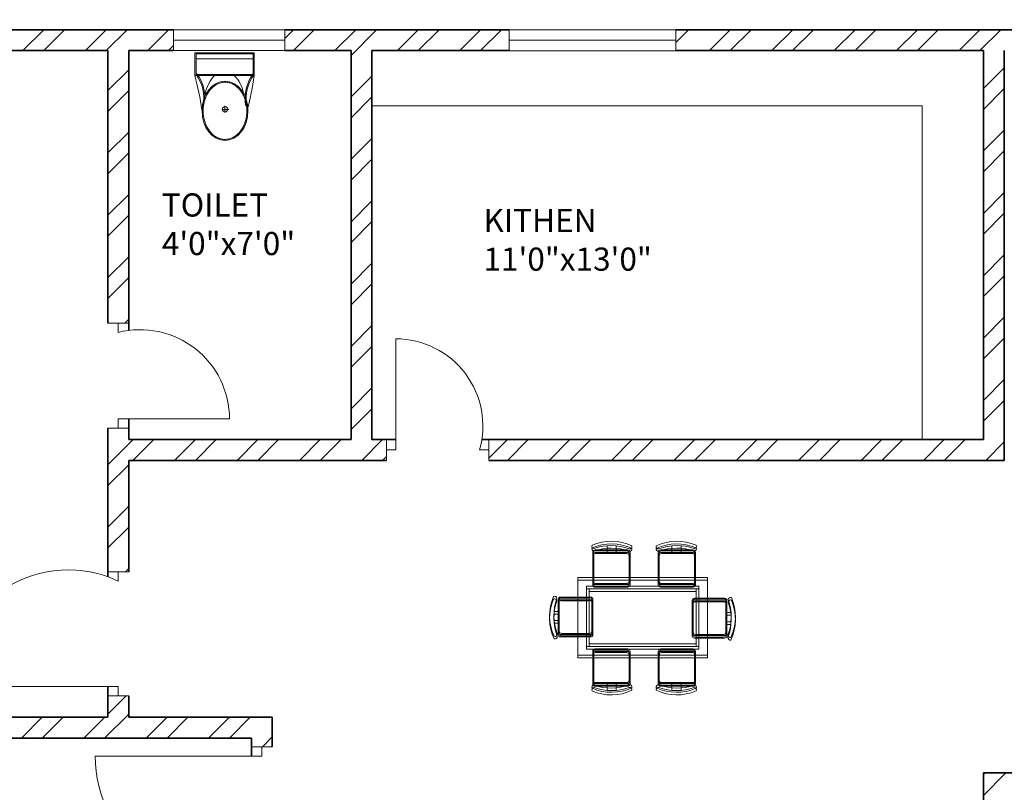
# Model space of a CAD drawing. Units: inches. Extents: x 1885 to 2748, y 783 to 2421.
# Tile 49 of 117: x 2098 to 2311, y 1683 to 1850. Entities that reach past the tile are written whole.
import ezdxf

# ---------------------------------------------------------------- set-up
doc = ezdxf.new("R2010")
doc.units = ezdxf.units.IN
for name, color, linetype, lineweight in [('A-AREA-IDEN', 7, 'Continuous', 18), ('A-DOOR', 31, 'Continuous', 18), ('A-FLOR-CASE', 9, 'Continuous', 18), ('A-FLOR-FIXT', 8, 'Continuous', 18), ('A-FURN', 8, 'Continuous', 13), ('A-GLAZ', 181, 'Continuous', 18), ('A-WALL', 7, 'Continuous', 35)]:
    doc.layers.add(name, color=color, linetype=linetype, lineweight=lineweight)
doc.layers.add('A-WALL-PATT', color=85, linetype='Continuous', lineweight=13, true_color=0x58ba48)
doc.styles.get("Standard").update_dxf_attribs({"font": 'arial.ttf'})

# ---------------------------------------------------------------- blocks, each defined once
blk = doc.blocks.new('A$C31115884')
for p, q in [((257.5, 466.4), (257.5, 523.2)), ((283.1, 497.7), (223.4, 497.7)), ((0, 200), (0, 0)), ((520, 200), (0, 200)), ((10, 190), (10, 10)), ((510, 190), (10, 190)), ((510, 10), (510, 190)), ((520, 0), (520, 200)), ((510, 54.5), (0, 54.5)), ((10, 10), (510, 10)), ((0, 0), (520, 0))]:
    blk.add_line(p, q)
blk.add_circle((255.6, 496.4), 23.6)
for centre, radius, start, end in [((2777.7, -204.6), 2807, 165.4549, 171.71327), ((-294.5, 403.3), 364.7, 324.20913, 9.34987), ((-294.5, 403.3), 374.7, 324.20913, 9.34987), ((805.8, 403.3), 364.7, 170.65013, 215.79087), ((3237, 905), 2807, 188.28673, 194.5451), ((383.6, 406.2), 293.5, 190.27735, 224.15636), ((139.5, 406.2), 293.5, 315.84364, 2.65635), ((805.8, 403.3), 374.7, 179.20365, 215.79087)]:
    blk.add_arc(centre, radius, start, end)
blk.add_ellipse((256.2, 509.9), major_axis=(0, -260.7), ratio=0.772727)
blk.add_open_spline([(256.2, 259.2), (263.1, 259.2), (270, 259.7), (287.8, 262.3), (298.7, 265.1), (319.9, 273.1), (330.2, 278.4), (350.1, 291.1), (359.7, 298.7), (377.7, 315.9), (386.2, 325.5), (401.7, 346.6), (408.8, 358.1), (421.3, 382.5), (426.8, 395.5), (435.9, 422.4), (439.5, 436.4), (444.8, 465.1), (446.5, 479.7), (447.9, 509.2), (447.6, 524), (445, 553.3), (442.7, 567.8), (436.3, 596), (432.1, 609.7), (421.9, 636), (416, 648.6), (402.5, 672.1), (395, 683), (378.6, 703), (369.8, 712.1), (351.1, 728), (341.3, 734.8), (320.9, 746.2), (310.4, 750.7), (288.9, 757.3), (278, 759.4), (256, 761), (245, 760.6), (223.1, 757.2), (212.3, 754.3), (191.1, 746.1), (180.8, 740.7), (160.9, 727.8), (151.4, 720.1), (133.5, 702.7), (125.1, 693), (109.6, 671.7), (102.6, 660.2), (90.2, 635.7), (84.9, 622.7), (76, 595.6), (72.4, 581.6), (67.2, 552.9), (65.6, 538.2), (64.4, 508.8), (64.8, 494), (67.5, 464.7), (69.9, 450.2), (76.6, 422), (80.8, 408.3), (91.1, 382.2), (97.2, 369.7), (110.8, 346.3), (118.4, 335.4), (134.8, 315.6), (143.7, 306.7), (162.4, 290.9), (172.3, 284.2), (192.8, 273), (203.3, 268.6), (224.8, 262.2), (235.8, 260.2), (249.9, 259.3), (253, 259.2), (256.2, 259.2)], degree=3, knots=[0, 0, 0, 0, 0.110105, 0.110105, 0.285049, 0.285049, 0.459994, 0.459994, 0.634938, 0.634938, 0.809882, 0.809882, 0.984827, 0.984827, 1.159771, 1.159771, 1.334715, 1.334715, 1.50966, 1.50966, 1.684604, 1.684604, 1.859549, 1.859549, 2.034493, 2.034493, 2.209437, 2.209437, 2.384382, 2.384382, 2.559326, 2.559326, 2.73427, 2.73427, 2.909215, 2.909215, 3.084159, 3.084159, 3.259103, 3.259103, 3.434048, 3.434048, 3.608992, 3.608992, 3.783936, 3.783936, 3.958881, 3.958881, 4.133825, 4.133825, 4.30877, 4.30877, 4.483714, 4.483714, 4.658658, 4.658658, 4.833603, 4.833603, 5.008547, 5.008547, 5.183491, 5.183491, 5.358436, 5.358436, 5.53338, 5.53338, 5.708324, 5.708324, 5.883269, 5.883269, 6.058213, 6.058213, 6.233158, 6.233158, 6.283185, 6.283185, 6.283185, 6.283185])
blk = doc.blocks.new('WIN-24')
for p, q in [((0, 4.5), (0, 0)), ((0, 4.5), (24, 4.5)), ((24, 2.25), (24, 4.5)), ((24, 4.5), (24, 0)), ((0, 0), (0, 2.25)), ((0, 2.25), (24, 2.25)), ((24, 0), (0, 0))]:
    blk.add_line(p, q)
blk = doc.blocks.new('WIN-36-ALT')
for p, q in [((0, 36), (4.5, 36)), ((0, 36), (0, 0)), ((4.5, 36), (2.25, 36)), ((2.25, 36), (2.25, 0)), ((4.5, 0), (4.5, 36)), ((4.5, 0), (0, 0)), ((2.25, 0), (4.5, 0))]:
    blk.add_line(p, q)

msp = doc.modelspace()

# ---------------------------------------------------------------- hatches: boundary and pattern name
at = {"layer": 'A-WALL-PATT'}
h = msp.add_hatch(dxfattribs=at)
h.set_pattern_fill('ANSI32', color=256)
h.paths.add_polyline_path([(2007.77, 2318.01), (1980.77, 2318.01), (1980.77, 2281.22), (1985.27, 2281.22), (1985.27, 2313.51), (2007.77, 2313.51), (2007.77, 2315.76)])
h.paths.add_polyline_path([(2094.32, 2318.01), (2067.77, 2318.01), (2067.77, 2313.51), (2094.32, 2313.51), (2094.32, 2315.76)])
h.paths.add_polyline_path([(2131.37, 2315.76), (2131.37, 2318.01), (2131.19, 2318.01), (2112.61, 2318.01), (2112.61, 2313.51), (2117.27, 2313.51), (2117.27, 2255.2), (2121.77, 2255.2), (2121.77, 2313.51), (2131.37, 2313.51)])
h.paths.add_polyline_path([(2190.51, 2318.01), (2155.37, 2318.01), (2155.37, 2313.51), (2169.77, 2313.51), (2169.77, 2229.51), (2121.77, 2229.51), (2121.77, 2233.45), (2119.52, 2233.45), (2117.27, 2233.45), (2117.27, 2201.1), (2121.77, 2201.1), (2121.77, 2225.01), (2169.77, 2225.01), (2169.77, 2165.01), (2306.27, 2165.01), (2306.27, 2066.01), (2310.77, 2066.01), (2344.27, 2066.01), (2486.27, 2066.01), (2486.27, 1886.01), (2483.02, 1886.01), (2483.02, 1881.51), (2486.27, 1881.51), (2486.27, 1880.68), (2490.77, 1880.68), (2490.77, 2070.51), (2344.27, 2070.51), (2310.77, 2070.51), (2310.77, 2165.01), (2310.77, 2173.64), (2308.52, 2173.64), (2306.27, 2173.64), (2306.27, 2169.51), (2174.27, 2169.51), (2174.27, 2313.51), (2190.51, 2313.51), (2190.51, 2315.76)])
h.paths.add_polyline_path([(1985.27, 2221.22), (1980.77, 2221.22), (1980.77, 2165.01), (1992.77, 2165.01), (1992.77, 2141.93), (1997.27, 2141.93), (1997.27, 2165.01), (2117.27, 2165.01), (2117.27, 2163.13), (2121.77, 2163.13), (2121.77, 2172.73), (2119.52, 2172.73), (2117.27, 2172.73), (2117.27, 2169.51), (1985.27, 2169.51)])
h.paths.add_polyline_path([(1997.27, 2105.93), (1992.77, 2105.93), (1992.77, 2070.51), (2016.77, 2070.51), (2016.77, 2059.12), (2019.02, 2059.12), (2021.27, 2059.12), (2021.27, 2070.51), (2117.27, 2070.51), (2117.27, 2022.51), (2114.42, 2022.51), (2114.42, 2018.01), (2123.63, 2018.01), (2123.63, 2020.26), (2123.63, 2022.51), (2121.77, 2022.51), (2121.77, 2142.59), (2119.52, 2142.59), (2117.27, 2142.59), (2117.27, 2075.01), (1997.27, 2075.01)])
h.paths.add_polyline_path([(2092.03, 2020.26), (2092.03, 2022.51), (2021.27, 2022.51), (2021.27, 2035.12), (2016.77, 2035.12), (2016.77, 2018.01), (2016.77, 1978.78), (2021.27, 1978.78), (2021.27, 2018.01), (2092.03, 2018.01)])
h.paths.add_polyline_path([(2260.94, 2022.51), (2153.1, 2022.51), (2153.1, 2020.26), (2153.1, 2018.01), (2155.27, 2018.01), (2155.27, 1886.01), (2107.63, 1886.01), (2107.63, 1881.51), (2182.91, 1881.51), (2182.91, 1883.76), (2182.91, 1886.01), (2159.77, 1886.01), (2159.77, 2018.01), (2260.94, 2018.01), (2260.94, 2020.26)])
h.paths.add_polyline_path([(2047.63, 1883.76), (2047.63, 1886.01), (2021.27, 1886.01), (2021.27, 1918.78), (2019.02, 1918.78), (2016.77, 1918.78), (2016.77, 1881.51), (2047.63, 1881.51)])
h.paths.add_polyline_path([(2306.36, 1883.76), (2306.36, 1886.01), (2296.27, 1886.01), (2296.27, 1982.01), (2316.54, 1982.01), (2316.54, 1984.26), (2316.54, 1986.51), (2296.27, 1986.51), (2296.27, 2022.51), (2289.28, 2022.51), (2289.28, 2018.01), (2291.77, 2018.01), (2291.77, 1886.01), (2242.91, 1886.01), (2242.91, 1881.51), (2306.36, 1881.51)], flags=17)
h.paths.add_polyline_path([(1985.27, 1843.01), (2021.6, 1843.01), (2021.53, 1845.44), (2021.48, 1847.51), (1980.77, 1847.51), (1980.77, 1809.45), (1985.27, 1809.45)])
h.paths.add_polyline_path([(2131.48, 1845.26), (2131.48, 1847.51), (2081.53, 1847.51), (2081.53, 1843.01), (2117.27, 1843.01), (2117.27, 1784.15), (2119.52, 1784.15), (2121.77, 1784.15), (2121.77, 1843.01), (2131.48, 1843.01)])
h.paths.add_polyline_path([(2203.89, 1847.51), (2155.48, 1847.51), (2155.48, 1843.01), (2169.77, 1843.01), (2169.77, 1759.01), (2121.77, 1759.01), (2121.77, 1761.46), (2117.27, 1761.46), (2117.27, 1730.43), (2121.77, 1730.43), (2121.77, 1754.51), (2177.42, 1754.51), (2177.42, 1756.76), (2177.42, 1759.01), (2174.27, 1759.01), (2174.27, 1843.01), (2203.89, 1843.01)])
h.paths.add_polyline_path([(2335.55, 1845.26), (2335.55, 1847.51), (2239.89, 1847.51), (2239.89, 1843.01), (2306.27, 1843.01), (2306.27, 1759.01), (2199.49, 1759.01), (2199.49, 1754.51), (2310.77, 1754.51), (2310.77, 1843.01), (2335.55, 1843.01)])
h.paths.add_polyline_path([(2348.77, 2022.51), (2344.27, 2022.51), (2344.27, 1986.51), (2341.68, 1986.51), (2341.68, 1982.01), (2344.27, 1982.01), (2344.27, 1886.01), (2330.36, 1886.01), (2330.36, 1881.51), (2361.63, 1881.51), (2361.63, 1883.76), (2361.63, 1886.01), (2348.77, 1886.01)], flags=17)
h.paths.add_polyline_path([(2283.25, 2315.76), (2283.25, 2318.01), (2238.51, 2318.01), (2238.51, 2313.51), (2283.25, 2313.51)], flags=17)
h.paths.add_polyline_path([(2363.27, 2348.01), (2388.68, 2348.01), (2388.68, 2350.26), (2388.68, 2352.51), (2358.77, 2352.51), (2358.77, 2348.01), (2358.77, 2318.01), (2344.48, 2318.01), (2344.48, 2313.51), (2358.77, 2313.51), (2358.77, 2229.51), (2310.77, 2229.51), (2310.77, 2231.95), (2306.27, 2231.95), (2306.27, 2205.61), (2310.77, 2205.61), (2310.77, 2225.01), (2358.77, 2225.01), (2358.77, 2211.51), (2452.33, 2211.51), (2452.33, 2213.76), (2452.33, 2216.01), (2363.27, 2216.01), (2363.27, 2318.01)])
h.paths.add_polyline_path([(2310.77, 2313.51), (2320.48, 2313.51), (2320.48, 2315.76), (2320.48, 2318.01), (2302.73, 2318.01), (2302.73, 2313.51), (2306.27, 2313.51), (2306.27, 2251.08), (2310.77, 2251.08)], flags=17)
h.paths.add_polyline_path([(2490.77, 2352.51), (2486.27, 2352.51), (2448.68, 2352.51), (2448.68, 2348.01), (2486.27, 2348.01), (2486.27, 2318.01), (2486.27, 2216.01), (2481.78, 2216.01), (2481.78, 2211.51), (2486.27, 2211.51), (2486.27, 2165.01), (2493.29, 2165.01), (2493.29, 2167.26), (2493.29, 2169.51), (2490.77, 2169.51), (2490.77, 2313.51), (2494.43, 2313.51), (2494.43, 2318.01), (2490.77, 2318.01)])
h.paths.add_polyline_path([(2534.65, 2318.01), (2515.69, 2318.01), (2515.69, 2313.51), (2534.65, 2313.51), (2534.65, 2315.76)])
h.paths.add_polyline_path([(2618.27, 2318.01), (2594.65, 2318.01), (2594.65, 2313.51), (2613.77, 2313.51), (2613.77, 2281.71), (2618.27, 2281.71)])
h.paths.add_polyline_path([(2618.27, 2221.71), (2613.77, 2221.71), (2613.77, 2169.51), (2554.02, 2169.51), (2554.02, 2165.01), (2613.77, 2165.01), (2613.77, 2152.88), (2618.27, 2152.88)])
h.paths.add_polyline_path([(2618.27, 2128.88), (2616.02, 2128.88), (2613.77, 2128.88), (2613.77, 2117.01), (2529.77, 2117.01), (2529.77, 2165.01), (2532.85, 2165.01), (2532.85, 2169.51), (2522.87, 2169.51), (2522.87, 2165.01), (2525.27, 2165.01), (2525.27, 2117.01), (2525.27, 2112.51), (2525.27, 2108.58), (2529.77, 2108.58), (2529.77, 2112.51), (2613.77, 2112.51), (2613.77, 2080.19), (2618.27, 2080.19)])
h.paths.add_polyline_path([(2618.27, 2044.19), (2616.02, 2044.19), (2613.77, 2044.19), (2613.77, 2015.51), (2529.77, 2015.51), (2529.77, 2088.58), (2527.52, 2088.58), (2525.27, 2088.58), (2525.27, 2011.01), (2613.77, 2011.01), (2613.77, 1956.75), (2618.27, 1956.75)])
h.paths.add_polyline_path([(2618.27, 1881.51), (2618.27, 1896.75), (2613.77, 1896.75), (2613.77, 1881.51), (2613.77, 1847.51), (2592.71, 1847.51), (2592.71, 1843.01), (2613.77, 1843.01), (2613.77, 1765.01), (2613.77, 1760.51), (2609.62, 1760.51), (2609.62, 1756.01), (2613.77, 1756.01), (2613.77, 1660.01), (2608.54, 1660.01), (2608.54, 1655.51), (2613.77, 1655.51), (2613.77, 1508.16), (2618.27, 1508.16)])
h.paths.add_polyline_path([(2565.77, 1843.01), (2569, 1843.01), (2569, 1847.51), (2490.77, 1847.51), (2490.77, 1849.7), (2488.52, 1849.7), (2486.27, 1849.7), (2486.27, 1847.51), (2477.27, 1847.51), (2477.27, 1838.51), (2477.27, 1821.49), (2486.27, 1821.49), (2486.27, 1838.51), (2561.27, 1838.51), (2561.27, 1765.01), (2486.27, 1765.01), (2486.27, 1786.16), (2477.27, 1786.16), (2477.27, 1765.01), (2477.27, 1756.01), (2486.27, 1756.01), (2565.77, 1756.01), (2585.62, 1756.01), (2585.62, 1758.26), (2585.62, 1760.51), (2565.77, 1760.51), (2565.77, 1765.01)])
h.paths.add_polyline_path([(2486.27, 1651.01), (2561.27, 1651.01), (2561.27, 1567.01), (2486.27, 1567.01), (2486.27, 1591.32), (2477.27, 1591.32), (2477.27, 1567.01), (2477.27, 1558.01), (2477.27, 1555.44), (2481.77, 1555.44), (2481.77, 1558.01), (2568.65, 1558.01), (2568.65, 1560.26), (2568.65, 1562.51), (2565.77, 1562.51), (2565.77, 1655.51), (2584.54, 1655.51), (2584.54, 1657.76), (2584.54, 1660.01), (2565.77, 1660.01), (2486.27, 1660.01), (2477.27, 1660.01), (2477.27, 1651.01), (2477.27, 1632.99), (2486.27, 1632.99)])
h.paths.add_polyline_path([(2449.97, 1883.76), (2449.97, 1886.01), (2421.63, 1886.01), (2421.63, 1881.51), (2449.97, 1881.51)], flags=17)
h.paths.add_polyline_path([(2447.27, 1847.51), (2395.55, 1847.51), (2395.55, 1843.01), (2442.77, 1843.01), (2442.77, 1809.27), (2447.27, 1809.27)])
h.paths.add_polyline_path([(1985.27, 1749.45), (1980.77, 1749.45), (1980.77, 1694.5), (1985.27, 1694.5), (1985.27, 1694.51), (1986.9, 1694.51), (1986.9, 1697.78), (1986.9, 1699.01), (1985.27, 1699.01)])
h.paths.add_polyline_path([(2152.77, 1699.01), (2121.77, 1699.01), (2121.77, 1703.67), (2119.52, 1703.67), (2117.27, 1703.67), (2117.27, 1699.01), (2009.22, 1699.01), (2009.22, 1694.51), (2148.27, 1694.51), (2148.27, 1692.63), (2152.77, 1692.63)])
h.paths.add_polyline_path([(2016.27, 1694.51), (2011.77, 1694.51), (2011.77, 1558.01), (2040.81, 1558.01), (2040.81, 1560.26), (2040.81, 1562.51), (2016.27, 1562.51)])
h.paths.add_polyline_path([(2152.77, 1663.02), (2150.52, 1663.02), (2148.27, 1663.02), (2148.27, 1562.51), (2100.81, 1562.51), (2100.81, 1558.01), (2165.12, 1558.01), (2165.12, 1560.26), (2165.12, 1562.51), (2152.77, 1562.51), (2152.77, 1610.51), (2224.77, 1610.51), (2224.77, 1607.99), (2229.27, 1607.99), (2229.27, 1615.01), (2152.77, 1615.01)])
h.paths.add_polyline_path([(2238.61, 1560.26), (2238.61, 1562.51), (2229.27, 1562.51), (2229.27, 1588.76), (2227.02, 1588.76), (2224.77, 1588.77), (2224.77, 1562.51), (2189.12, 1562.51), (2189.12, 1558.01), (2238.61, 1558.01)])
h.paths.add_polyline_path([(2336.02, 1560.26), (2336.02, 1562.51), (2310.77, 1562.51), (2310.77, 1656.35), (2308.52, 1656.35), (2306.27, 1656.35), (2306.27, 1562.51), (2286.61, 1562.51), (2286.61, 1558.01), (2336.02, 1558.01)])
h.paths.add_polyline_path([(2447.27, 1690.97), (2445.02, 1690.97), (2442.77, 1690.97), (2442.77, 1687.01), (2306.27, 1687.01), (2306.27, 1680.75), (2310.77, 1680.75), (2310.77, 1682.51), (2442.77, 1682.51), (2442.77, 1562.51), (2396.02, 1562.51), (2396.02, 1558.01), (2447.27, 1558.01)])
h.paths.add_polyline_path([(2447.27, 1749.27), (2445.02, 1749.27), (2442.77, 1749.27), (2442.77, 1717.23), (2447.27, 1717.23)])
h.paths.add_polyline_path([(2044.67, 1521.76), (2044.67, 1524.01), (2007.27, 1524.01), (2007.27, 1503.49), (2009.52, 1503.49), (2011.77, 1503.49), (2011.77, 1519.51), (2044.67, 1519.51)])
h.paths.add_polyline_path([(2177.97, 1521.76), (2177.97, 1524.01), (2104.67, 1524.01), (2104.67, 1519.51), (2145.77, 1519.51), (2145.77, 1387.51), (2143.37, 1387.51), (2143.37, 1383.01), (2251.59, 1383.01), (2251.59, 1385.26), (2251.59, 1387.51), (2150.27, 1387.51), (2150.27, 1519.51), (2177.97, 1519.51)])
h.paths.add_polyline_path([(2298.7, 1524.01), (2237.97, 1524.01), (2237.97, 1519.51), (2282.27, 1519.51), (2282.27, 1387.51), (2279.68, 1387.51), (2279.68, 1383.01), (2286.77, 1383.01), (2286.77, 1419.01), (2312.45, 1419.01), (2312.45, 1421.26), (2312.45, 1423.51), (2286.77, 1423.51), (2286.77, 1519.51), (2298.7, 1519.51), (2298.7, 1521.72)], flags=17)
h.paths.add_polyline_path([(2361.9, 1521.76), (2361.9, 1524.01), (2322.7, 1524.01), (2322.7, 1519.51), (2334.77, 1519.51), (2334.77, 1423.51), (2331.93, 1423.51), (2331.93, 1419.01), (2334.77, 1419.01), (2334.77, 1387.51), (2334.77, 1383.23), (2339.27, 1383.23), (2339.27, 1387.51), (2339.27, 1519.51), (2361.9, 1519.51)], flags=17)
h.paths.add_polyline_path([(2447.27, 1521.76), (2447.27, 1524.01), (2421.9, 1524.01), (2421.9, 1519.51), (2447.27, 1519.51)], flags=17)
h.paths.add_polyline_path([(2481.77, 1529.6), (2479.52, 1529.6), (2477.27, 1529.6), (2477.27, 1524.01), (2474.49, 1524.01), (2474.49, 1519.51), (2477.27, 1519.51), (2477.27, 1334.51), (2296.77, 1334.51), (2296.77, 1240.51), (2160.27, 1240.51), (2160.27, 1180.51), (2112.27, 1180.51), (2112.27, 1207.69), (2110.02, 1207.69), (2107.77, 1207.69), (2107.77, 1171.61), (2112.27, 1171.61), (2112.27, 1176.01), (2160.27, 1176.01), (2160.27, 1092.01), (2144.22, 1092.01), (2144.22, 1087.51), (2189.5, 1087.51), (2189.5, 1089.76), (2189.5, 1092.01), (2164.77, 1092.01), (2164.77, 1236.01), (2296.77, 1236.01), (2296.77, 1231.91), (2301.27, 1231.91), (2301.27, 1330.01), (2481.77, 1330.01), (2481.77, 1387.51)])
h.paths.add_polyline_path([(2618.27, 1448.16), (2613.77, 1448.16), (2613.77, 1382.51), (2529.77, 1382.51), (2525.27, 1382.51), (2525.27, 1307.06), (2529.77, 1307.06), (2529.77, 1378.01), (2613.77, 1378.01), (2613.77, 1354.99), (2618.27, 1354.99)])
h.paths.add_polyline_path([(2618.27, 1318.99), (2613.77, 1318.99), (2613.77, 1281.01), (2529.77, 1281.01), (2529.77, 1283.79), (2527.52, 1283.79), (2525.27, 1283.79), (2525.27, 1228.51), (2516.79, 1228.51), (2516.79, 1224.01), (2533.48, 1224.01), (2533.48, 1226.26), (2533.48, 1228.51), (2529.77, 1228.51), (2529.77, 1276.51), (2613.77, 1276.51), (2613.77, 1266.02), (2618.27, 1266.02)])
h.paths.add_polyline_path([(2618.27, 1134.96), (2613.77, 1134.96), (2613.77, 1092.01), (2594.54, 1092.01), (2594.54, 1087.51), (2618.27, 1087.51)])
h.paths.add_polyline_path([(2534.54, 1092.01), (2509.77, 1092.01), (2509.77, 1087.51), (2534.54, 1087.51), (2534.54, 1089.76)])
h.paths.add_polyline_path([(2481.27, 1224.01), (2484.12, 1224.01), (2484.12, 1226.26), (2484.12, 1228.51), (2476.77, 1228.51), (2476.77, 1198.51), (2471.61, 1198.51), (2471.61, 1194.01), (2476.77, 1194.01), (2476.77, 1062.01), (2436.89, 1062.01), (2436.89, 1057.51), (2476.77, 1057.51), (2481.27, 1057.51), (2481.27, 1062.01), (2481.27, 1087.51), (2485.35, 1087.51), (2485.35, 1089.76), (2485.35, 1092.01), (2481.27, 1092.01), (2481.27, 1117.51)])
h.paths.add_polyline_path([(2439.9, 1198.51), (2349.27, 1198.51), (2349.27, 1194.01), (2349.27, 1180.51), (2301.27, 1180.51), (2301.27, 1201.9), (2299.02, 1201.9), (2296.77, 1201.9), (2296.77, 1172.34), (2299.02, 1172.34), (2301.27, 1172.34), (2301.27, 1176.01), (2349.27, 1176.01), (2349.27, 1092.01), (2334.45, 1092.01), (2334.45, 1087.51), (2349.27, 1087.51), (2349.27, 1057.51), (2353.77, 1057.51), (2376.89, 1057.51), (2376.89, 1059.76), (2376.89, 1062.01), (2353.77, 1062.01), (2353.77, 1087.51), (2353.77, 1180.51), (2353.77, 1194.01), (2439.9, 1194.01), (2439.9, 1196.26)])
h.paths.add_polyline_path([(2270.6, 1089.76), (2270.6, 1092.01), (2249.5, 1092.01), (2249.5, 1087.51), (2270.6, 1087.51)], flags=17)
h.paths.add_polyline_path([(2310.45, 1092.01), (2301.27, 1092.01), (2301.27, 1153.29), (2296.77, 1153.29), (2296.77, 1092.01), (2293.79, 1092.01), (2293.79, 1087.51), (2310.45, 1087.51), (2310.45, 1089.76)], flags=17)
h.paths.add_polyline_path([(2112.27, 1150.33), (2110.02, 1150.33), (2107.77, 1150.33), (2107.77, 1092.01), (2104.47, 1092.01), (2104.47, 1087.51), (2120.22, 1087.51), (2120.22, 1089.76), (2120.22, 1092.01), (2112.27, 1092.01)])
h.paths.add_polyline_path([(2082.17, 1092.01), (2058.14, 1092.01), (2058.14, 1087.51), (2082.17, 1087.51), (2082.17, 1089.76)])
h.paths.add_polyline_path([(1975.77, 1145.64), (1971.27, 1145.64), (1971.27, 1087.51), (1980.77, 1087.51), (1998.14, 1087.51), (1998.14, 1089.76), (1998.14, 1092.01), (1985.27, 1092.01), (1975.77, 1092.01)])
h.paths.add_polyline_path([(2112.27, 1244.38), (2110.02, 1244.38), (2107.77, 1244.38), (2107.77, 1240.51), (1992.27, 1240.51), (1992.27, 1271.01), (1987.77, 1271.01), (1987.77, 1240.51), (1980.77, 1240.51), (1975.77, 1240.51), (1971.27, 1240.51), (1971.27, 1205.64), (1975.77, 1205.64), (1975.77, 1236.01), (2107.77, 1236.01), (2107.77, 1233.44), (2112.27, 1233.44), (2112.27, 1236.01)])
h.paths.add_polyline_path([(2112.27, 1383.01), (2114.78, 1383.01), (2114.78, 1385.26), (2114.78, 1387.51), (2102.48, 1387.51), (2102.48, 1383.01), (2107.77, 1383.01), (2107.77, 1335.01), (2011.77, 1335.01), (2011.77, 1349.94), (2007.27, 1349.94), (2007.27, 1335.01), (1987.77, 1335.01), (1987.77, 1330.51), (1987.77, 1307.01), (1992.27, 1307.01), (1992.27, 1330.51), (2007.27, 1330.51), (2107.77, 1330.51), (2107.77, 1264.71), (2112.27, 1264.71)])
h.paths.add_polyline_path([(2077.86, 1387.51), (2011.77, 1387.51), (2011.77, 1390.04), (2009.52, 1390.04), (2007.27, 1390.04), (2007.27, 1373.94), (2011.77, 1373.94), (2011.77, 1383.01), (2077.86, 1383.01)])
h.paths.add_polyline_path([(2011.77, 1443.49), (2007.27, 1443.49), (2007.27, 1410.25), (2011.77, 1410.25)])

# ---------------------------------------------------------------- linework, layer by layer
at = {"layer": 'A-DOOR'}
for p, q in [((2121.77, 1784.15), (2117.27, 1784.15)), ((2117.27, 1784.15), (2119.52, 1784.15)), ((2119.52, 1784.15), (2119.52, 1782.15)), ((2179.42, 1756.76), (2179.42, 1780.76)), ((2119.52, 1761.46), (2119.52, 1763.46)), ((2119.52, 1763.46), (2143.52, 1763.46)), ((2121.77, 1761.46), (2117.27, 1761.46)), ((2117.27, 1761.46), (2119.52, 1761.46)), ((2177.42, 1759.01), (2177.42, 1754.51)), ((2199.49, 1759.01), (2199.49, 1754.51)), ((2177.42, 1754.51), (2177.42, 1756.76)), ((2177.42, 1756.76), (2179.42, 1756.76)), ((2199.49, 1756.76), (2197.49, 1756.76)), ((2199.49, 1754.51), (2199.49, 1756.76)), ((2117.27, 1730.43), (2121.77, 1730.43)), ((2121.77, 1730.43), (2119.52, 1730.43)), ((2119.52, 1730.43), (2119.52, 1728.43)), ((2119.52, 1705.67), (2083.52, 1705.67)), ((2119.52, 1703.67), (2119.52, 1705.67)), ((2117.27, 1703.67), (2121.77, 1703.67)), ((2121.77, 1703.67), (2119.52, 1703.67)), ((2148.27, 1692.63), (2152.77, 1692.63)), ((2152.77, 1692.63), (2150.52, 1692.63)), ((2150.52, 1692.63), (2150.52, 1690.63)), ((2150.52, 1690.63), (2114.52, 1690.63))]:
    msp.add_line(p, q, dxfattribs=at)
for centre, radius, start, end in [((2124.25, 1763.46), 19.28, 0, 104.1812), ((2179.42, 1761.96), 18.8, 343.9381, 90), ((2108.72, 1705.67), 25.19, 64.6047, 180), ((2141.64, 1690.63), 27.11, 180, 289.1371)]:
    msp.add_arc(centre, radius, start, end, dxfattribs=at)
at = {"layer": 'A-FLOR-CASE'}
for p, q in [((2174.27, 1831.09), (2293.01, 1831.09)), ((2293.01, 1831.09), (2293.01, 1759.01))]:
    msp.add_line(p, q, dxfattribs=at)
at = {"layer": 'A-FURN'}
for points in [[(2222.21, 1735.47, -0.175809), (2229.82, 1735.42, 0.578392), (2230.4, 1736.05, 0.214524), (2221.8, 1736.17, 0.552014), (2222.21, 1735.47, -0.065079)], [(2222.21, 1735.47, -0.175809), (2229.82, 1735.42, 0.578392), (2230.4, 1736.05, 0.214524), (2221.8, 1736.17, 0.552014), (2222.21, 1735.47, -0.065079)], [(2222.21, 1734.92, -0.175809), (2229.82, 1734.86, 0.578392), (2230.4, 1735.49, 0.214524), (2221.8, 1735.61, 0.552014), (2222.21, 1734.92, -0.065079)], [(2222.21, 1734.92, -0.175809), (2229.82, 1734.86, 0.578392), (2230.4, 1735.49, 0.214524), (2221.8, 1735.61, 0.552014), (2222.21, 1734.92, -0.065079)], [(2236.23, 1735.42, -0.578392), (2235.65, 1736.05, -0.214524), (2244.25, 1736.17, -0.552014), (2243.84, 1735.47, 0.175809), (2236.23, 1735.42)], [(2236.23, 1735.42, -0.578392), (2235.65, 1736.05, -0.214524), (2244.25, 1736.17, -0.552014), (2243.84, 1735.47, 0.175809), (2236.23, 1735.42)], [(2236.23, 1734.86, -0.578392), (2235.65, 1735.49, -0.214524), (2244.25, 1735.61, -0.552014), (2243.84, 1734.92, 0.175809), (2236.23, 1734.86)], [(2236.23, 1734.86, -0.578392), (2235.65, 1735.49, -0.214524), (2244.25, 1735.61, -0.552014), (2243.84, 1734.92, 0.175809), (2236.23, 1734.86)], [(2229.5, 1735.17), (2222.43, 1735.17, 0.414214), (2221.93, 1734.67), (2221.93, 1728.18, 0.414214), (2222.43, 1727.68), (2229.5, 1727.68, 0.414214), (2229.99, 1728.18), (2229.99, 1734.67, 0.414214), (2229.5, 1735.17)], [(2229.5, 1735.17), (2222.43, 1735.17, 0.414214), (2221.93, 1734.67), (2221.93, 1728.18, 0.414214), (2222.43, 1727.68), (2229.5, 1727.68, 0.414214), (2229.99, 1728.18), (2229.99, 1734.67, 0.414214), (2229.5, 1735.17)], [(2229.5, 1734.61), (2222.43, 1734.61, 0.414214), (2221.93, 1734.12), (2221.93, 1727.62, 0.414214), (2222.43, 1727.12), (2229.5, 1727.12, 0.414214), (2229.99, 1727.62), (2229.99, 1734.12, 0.414214), (2229.5, 1734.61)], [(2229.5, 1734.61), (2222.43, 1734.61, 0.414214), (2221.93, 1734.12), (2221.93, 1727.62, 0.414214), (2222.43, 1727.12), (2229.5, 1727.12, 0.414214), (2229.99, 1727.62), (2229.99, 1734.12, 0.414214), (2229.5, 1734.61)], [(2227.01, 1735.17), (2227.01, 1736.06, -0.064759)], [(2227.01, 1735.17), (2227.01, 1736.06, -0.064759)], [(2227.01, 1734.61), (2227.01, 1735.5, -0.064759)], [(2227.01, 1734.61), (2227.01, 1735.5, -0.064759)], [(2243.62, 1735.17, -0.414214), (2244.11, 1734.67), (2244.11, 1728.18, -0.414214), (2243.62, 1727.68), (2236.55, 1727.68, -0.414214), (2236.06, 1728.18), (2236.06, 1734.67, -0.414214), (2236.55, 1735.17), (2243.62, 1735.17)], [(2243.62, 1735.17, -0.414214), (2244.11, 1734.67), (2244.11, 1728.18, -0.414214), (2243.62, 1727.68), (2236.55, 1727.68, -0.414214), (2236.06, 1728.18), (2236.06, 1734.67, -0.414214), (2236.55, 1735.17), (2243.62, 1735.17)], [(2243.62, 1734.61, -0.414214), (2244.11, 1734.12), (2244.11, 1727.62, -0.414214), (2243.62, 1727.12), (2236.55, 1727.12, -0.414214), (2236.06, 1727.62), (2236.06, 1734.12, -0.414214), (2236.55, 1734.61), (2243.62, 1734.61)], [(2243.62, 1734.61, -0.414214), (2244.11, 1734.12), (2244.11, 1727.62, -0.414214), (2243.62, 1727.12), (2236.55, 1727.12, -0.414214), (2236.06, 1727.62), (2236.06, 1734.12, -0.414214), (2236.55, 1734.61), (2243.62, 1734.61)], [(2239.03, 1735.17), (2239.03, 1736.06, 0.064759)], [(2239.03, 1735.17), (2239.03, 1736.06, 0.064759)], [(2239.03, 1734.61), (2239.03, 1735.5, 0.064759)], [(2239.03, 1734.61), (2239.03, 1735.5, 0.064759)], [(2214.24, 1717.09, -0.578392), (2213.61, 1716.51, -0.214524), (2213.49, 1725.11, -0.552014), (2214.18, 1724.7, 0.175809), (2214.24, 1717.09)], [(2214.24, 1717.09, -0.578392), (2213.61, 1716.51, -0.214524), (2213.49, 1725.11, -0.552014), (2214.18, 1724.7, 0.175809), (2214.24, 1717.09)], [(2214.24, 1716.53, -0.578392), (2213.61, 1715.95, -0.214524), (2213.49, 1724.55, -0.552014), (2214.18, 1724.14, 0.175809), (2214.24, 1716.53)], [(2214.24, 1716.53, -0.578392), (2213.61, 1715.95, -0.214524), (2213.49, 1724.55, -0.552014), (2214.18, 1724.14, 0.175809), (2214.24, 1716.53)], [(2214.49, 1724.48, -0.414214), (2214.98, 1724.98), (2221.48, 1724.98, -0.414214), (2221.98, 1724.48), (2221.98, 1717.41, -0.414214), (2221.48, 1716.92), (2214.98, 1716.92, -0.414214), (2214.49, 1717.41), (2214.49, 1724.48)], [(2214.49, 1724.48, -0.414214), (2214.98, 1724.98), (2221.48, 1724.98, -0.414214), (2221.98, 1724.48), (2221.98, 1717.41, -0.414214), (2221.48, 1716.92), (2214.98, 1716.92, -0.414214), (2214.49, 1717.41), (2214.49, 1724.48)], [(2214.49, 1723.92, -0.414214), (2214.98, 1724.42), (2221.48, 1724.42, -0.414214), (2221.98, 1723.92), (2221.98, 1716.85, -0.414214), (2221.48, 1716.36), (2214.98, 1716.36, -0.414214), (2214.49, 1716.85), (2214.49, 1723.92)], [(2214.49, 1723.92, -0.414214), (2214.98, 1724.42), (2221.48, 1724.42, -0.414214), (2221.98, 1723.92), (2221.98, 1716.85, -0.414214), (2221.48, 1716.36), (2214.98, 1716.36, -0.414214), (2214.49, 1716.85), (2214.49, 1723.92)], [(2250.89, 1724.24, 0.414214), (2250.39, 1724.73), (2243.89, 1724.73, 0.414214), (2243.4, 1724.24), (2243.4, 1717.17, 0.414214), (2243.89, 1716.68), (2250.39, 1716.68, 0.414214), (2250.89, 1717.17), (2250.89, 1724.24)], [(2250.89, 1724.24, 0.414214), (2250.39, 1724.73), (2243.89, 1724.73, 0.414214), (2243.4, 1724.24), (2243.4, 1717.17, 0.414214), (2243.89, 1716.68), (2250.39, 1716.68, 0.414214), (2250.89, 1717.17), (2250.89, 1724.24)], [(2250.89, 1723.68, 0.414214), (2250.39, 1724.17), (2243.89, 1724.17, 0.414214), (2243.4, 1723.68), (2243.4, 1716.61, 0.414214), (2243.89, 1716.12), (2250.39, 1716.12, 0.414214), (2250.89, 1716.61), (2250.89, 1723.68)], [(2250.89, 1723.68, 0.414214), (2250.39, 1724.17), (2243.89, 1724.17, 0.414214), (2243.4, 1723.68), (2243.4, 1716.61, 0.414214), (2243.89, 1716.12), (2250.39, 1716.12, 0.414214), (2250.89, 1716.61), (2250.89, 1723.68)], [(2251.19, 1724.46, -0.175809), (2251.13, 1716.85, 0.578392), (2251.77, 1716.27, 0.214524), (2251.88, 1724.86, 0.552014), (2251.19, 1724.46, -0.065079)], [(2251.19, 1724.46, -0.175809), (2251.13, 1716.85, 0.578392), (2251.77, 1716.27, 0.214524), (2251.88, 1724.86, 0.552014), (2251.19, 1724.46, -0.065079)], [(2251.19, 1723.9, -0.175809), (2251.13, 1716.29, 0.578392), (2251.77, 1715.71, 0.214524), (2251.88, 1724.31, 0.552014), (2251.19, 1723.9, -0.065079)], [(2251.19, 1723.9, -0.175809), (2251.13, 1716.29, 0.578392), (2251.77, 1715.71, 0.214524), (2251.88, 1724.31, 0.552014), (2251.19, 1723.9, -0.065079)], [(2214.49, 1719.9), (2213.59, 1719.9, 0.064759)], [(2214.49, 1719.9), (2213.59, 1719.9, 0.064759)], [(2250.89, 1719.65), (2251.78, 1719.65, -0.064759)], [(2250.89, 1719.65), (2251.78, 1719.65, -0.064759)], [(2214.49, 1719.34), (2213.59, 1719.34, 0.064759)], [(2214.49, 1719.34), (2213.59, 1719.34, 0.064759)], [(2250.89, 1719.09), (2251.78, 1719.09, -0.064759)], [(2250.89, 1719.09), (2251.78, 1719.09, -0.064759)], [(2229.5, 1706.28), (2222.43, 1706.28, -0.414214), (2221.93, 1706.77), (2221.93, 1713.27, -0.414214), (2222.43, 1713.77), (2229.5, 1713.77, -0.414214), (2229.99, 1713.27), (2229.99, 1706.77, -0.414214), (2229.5, 1706.28)], [(2229.5, 1706.28), (2222.43, 1706.28, -0.414214), (2221.93, 1706.77), (2221.93, 1713.27, -0.414214), (2222.43, 1713.77), (2229.5, 1713.77, -0.414214), (2229.99, 1713.27), (2229.99, 1706.77, -0.414214), (2229.5, 1706.28)], [(2229.5, 1705.72), (2222.43, 1705.72, -0.414214), (2221.93, 1706.22), (2221.93, 1712.71, -0.414214), (2222.43, 1713.21), (2229.5, 1713.21, -0.414214), (2229.99, 1712.71), (2229.99, 1706.22, -0.414214), (2229.5, 1705.72)], [(2229.5, 1705.72), (2222.43, 1705.72, -0.414214), (2221.93, 1706.22), (2221.93, 1712.71, -0.414214), (2222.43, 1713.21), (2229.5, 1713.21, -0.414214), (2229.99, 1712.71), (2229.99, 1706.22, -0.414214), (2229.5, 1705.72)], [(2243.62, 1706.28, 0.414214), (2244.11, 1706.77), (2244.11, 1713.27, 0.414214), (2243.62, 1713.77), (2236.55, 1713.77, 0.414214), (2236.06, 1713.27), (2236.06, 1706.77, 0.414214), (2236.55, 1706.28), (2243.62, 1706.28)], [(2243.62, 1706.28, 0.414214), (2244.11, 1706.77), (2244.11, 1713.27, 0.414214), (2243.62, 1713.77), (2236.55, 1713.77, 0.414214), (2236.06, 1713.27), (2236.06, 1706.77, 0.414214), (2236.55, 1706.28), (2243.62, 1706.28)], [(2243.62, 1705.72, 0.414214), (2244.11, 1706.22), (2244.11, 1712.71, 0.414214), (2243.62, 1713.21), (2236.55, 1713.21, 0.414214), (2236.06, 1712.71), (2236.06, 1706.22, 0.414214), (2236.55, 1705.72), (2243.62, 1705.72)], [(2243.62, 1705.72, 0.414214), (2244.11, 1706.22), (2244.11, 1712.71, 0.414214), (2243.62, 1713.21), (2236.55, 1713.21, 0.414214), (2236.06, 1712.71), (2236.06, 1706.22, 0.414214), (2236.55, 1705.72), (2243.62, 1705.72)], [(2229.82, 1706.03, -0.578392), (2230.4, 1705.4, -0.214524), (2221.8, 1705.28, -0.552014), (2222.21, 1705.97, 0.175809), (2229.82, 1706.03)], [(2229.82, 1706.03, -0.578392), (2230.4, 1705.4, -0.214524), (2221.8, 1705.28, -0.552014), (2222.21, 1705.97, 0.175809), (2229.82, 1706.03)], [(2229.82, 1705.47, -0.578392), (2230.4, 1704.84, -0.214524), (2221.8, 1704.72, -0.552014), (2222.21, 1705.42, 0.175809), (2229.82, 1705.47)], [(2229.82, 1705.47, -0.578392), (2230.4, 1704.84, -0.214524), (2221.8, 1704.72, -0.552014), (2222.21, 1705.42, 0.175809), (2229.82, 1705.47)], [(2227.01, 1706.28), (2227.01, 1705.39, 0.064759)], [(2227.01, 1706.28), (2227.01, 1705.39, 0.064759)], [(2227.01, 1705.72), (2227.01, 1704.83, 0.064759)], [(2227.01, 1705.72), (2227.01, 1704.83, 0.064759)], [(2243.84, 1705.97, -0.175809), (2236.23, 1706.03, 0.578392), (2235.65, 1705.4, 0.214524), (2244.25, 1705.28, 0.552014), (2243.84, 1705.97, -0.065079)], [(2243.84, 1705.97, -0.175809), (2236.23, 1706.03, 0.578392), (2235.65, 1705.4, 0.214524), (2244.25, 1705.28, 0.552014), (2243.84, 1705.97, -0.065079)], [(2243.84, 1705.42, -0.175809), (2236.23, 1705.47, 0.578392), (2235.65, 1704.84, 0.214524), (2244.25, 1704.72, 0.552014), (2243.84, 1705.42, -0.065079)], [(2243.84, 1705.42, -0.175809), (2236.23, 1705.47, 0.578392), (2235.65, 1704.84, 0.214524), (2244.25, 1704.72, 0.552014), (2243.84, 1705.42, -0.065079)], [(2239.03, 1706.28), (2239.03, 1705.39, -0.064759)], [(2239.03, 1706.28), (2239.03, 1705.39, -0.064759)], [(2239.03, 1705.72), (2239.03, 1704.83, -0.064759)], [(2239.03, 1705.72), (2239.03, 1704.83, -0.064759)]]:
    msp.add_lwpolyline(points, format="xyb", dxfattribs=at)
for points in [[(2222.43, 1734.95), (2229.27, 1734.95, -0.414214), (2229.77, 1734.45), (2229.77, 1728.4, -0.414214), (2229.27, 1727.9), (2222.43, 1727.9, -0.512069), (2222.16, 1728.4), (2222.16, 1734.45, -0.512069)], [(2222.43, 1734.95), (2229.27, 1734.95, -0.414214), (2229.77, 1734.45), (2229.77, 1728.4, -0.414214), (2229.27, 1727.9), (2222.43, 1727.9, -0.512069), (2222.16, 1728.4), (2222.16, 1734.45, -0.512069)], [(2222.43, 1734.39), (2229.27, 1734.39, -0.414214), (2229.77, 1733.89), (2229.77, 1727.84, -0.414214), (2229.27, 1727.35), (2222.43, 1727.35, -0.512069), (2222.16, 1727.84), (2222.16, 1733.89, -0.512069)], [(2222.43, 1734.39), (2229.27, 1734.39, -0.414214), (2229.77, 1733.89), (2229.77, 1727.84, -0.414214), (2229.27, 1727.34), (2222.43, 1727.34, -0.512069), (2222.16, 1727.84), (2222.16, 1733.89, -0.512069)], [(2243.62, 1734.95), (2236.77, 1734.95, 0.414214), (2236.28, 1734.45), (2236.28, 1728.4, 0.414214), (2236.77, 1727.9), (2243.62, 1727.9, 0.512069), (2243.89, 1728.4), (2243.89, 1734.45, 0.512069)], [(2243.62, 1734.95), (2236.77, 1734.95, 0.414214), (2236.28, 1734.45), (2236.28, 1728.4, 0.414214), (2236.77, 1727.9), (2243.62, 1727.9, 0.512069), (2243.89, 1728.4), (2243.89, 1734.45, 0.512069)], [(2243.62, 1734.39), (2236.77, 1734.39, 0.414214), (2236.28, 1733.89), (2236.28, 1727.84, 0.414214), (2236.77, 1727.35), (2243.62, 1727.35, 0.512069), (2243.89, 1727.84), (2243.89, 1733.89, 0.512069)], [(2243.62, 1734.39), (2236.77, 1734.39, 0.414214), (2236.28, 1733.89), (2236.28, 1727.84, 0.414214), (2236.77, 1727.34), (2243.62, 1727.34, 0.512069), (2243.89, 1727.84), (2243.89, 1733.89, 0.512069)], [(2214.71, 1724.48), (2214.71, 1717.64, 0.414214), (2215.21, 1717.14), (2221.26, 1717.14, 0.414214), (2221.75, 1717.64), (2221.75, 1724.48, 0.512069), (2221.26, 1724.75), (2215.21, 1724.75, 0.512069)], [(2214.71, 1724.48), (2214.71, 1717.64, 0.414214), (2215.21, 1717.14), (2221.26, 1717.14, 0.414214), (2221.75, 1717.64), (2221.75, 1724.48, 0.512069), (2221.26, 1724.75), (2215.21, 1724.75, 0.512069)], [(2214.71, 1723.92), (2214.71, 1717.08, 0.414214), (2215.21, 1716.58), (2221.26, 1716.58, 0.414214), (2221.75, 1717.08), (2221.75, 1723.92, 0.512069), (2221.26, 1724.19), (2215.21, 1724.19, 0.512069)], [(2214.71, 1723.92), (2214.71, 1717.08, 0.414214), (2215.21, 1716.58), (2221.26, 1716.58, 0.414214), (2221.75, 1717.08), (2221.75, 1723.92, 0.512069), (2221.26, 1724.19), (2215.21, 1724.19, 0.512069)], [(2250.66, 1724.24), (2250.66, 1717.39, -0.414214), (2250.17, 1716.9), (2244.11, 1716.9, -0.414214), (2243.62, 1717.39), (2243.62, 1724.24, -0.512069), (2244.11, 1724.51), (2250.17, 1724.51, -0.512069)], [(2250.66, 1724.24), (2250.66, 1717.39, -0.414214), (2250.17, 1716.9), (2244.11, 1716.9, -0.414214), (2243.62, 1717.39), (2243.62, 1724.24, -0.512069), (2244.11, 1724.51), (2250.17, 1724.51, -0.512069)], [(2250.66, 1723.68), (2250.66, 1716.83, -0.414214), (2250.17, 1716.34), (2244.11, 1716.34, -0.414214), (2243.62, 1716.83), (2243.62, 1723.68, -0.512069), (2244.11, 1723.95), (2250.17, 1723.95, -0.512069)], [(2250.66, 1723.68), (2250.66, 1716.83, -0.414214), (2250.17, 1716.34), (2244.11, 1716.34, -0.414214), (2243.62, 1716.83), (2243.62, 1723.68, -0.512069), (2244.11, 1723.95), (2250.17, 1723.95, -0.512069)], [(2222.43, 1706.5), (2229.27, 1706.5, 0.414214), (2229.77, 1707), (2229.77, 1713.05, 0.414214), (2229.27, 1713.55), (2222.43, 1713.55, 0.512069), (2222.16, 1713.05), (2222.16, 1707, 0.512069)], [(2222.43, 1706.5), (2229.27, 1706.5, 0.414214), (2229.77, 1707), (2229.77, 1713.05, 0.414214), (2229.27, 1713.55), (2222.43, 1713.55, 0.512069), (2222.16, 1713.05), (2222.16, 1707, 0.512069)], [(2222.43, 1705.94), (2229.27, 1705.94, 0.414214), (2229.77, 1706.44), (2229.77, 1712.49, 0.414214), (2229.27, 1712.99), (2222.43, 1712.99, 0.512069), (2222.16, 1712.49), (2222.16, 1706.44, 0.512069)], [(2222.43, 1705.94), (2229.27, 1705.94, 0.414214), (2229.77, 1706.44), (2229.77, 1712.49, 0.414214), (2229.27, 1712.99), (2222.43, 1712.99, 0.512069), (2222.16, 1712.49), (2222.16, 1706.44, 0.512069)], [(2243.62, 1706.5), (2236.77, 1706.5, -0.414214), (2236.28, 1707), (2236.28, 1713.05, -0.414214), (2236.77, 1713.55), (2243.62, 1713.55, -0.512069), (2243.89, 1713.05), (2243.89, 1707, -0.512069)], [(2243.62, 1706.5), (2236.77, 1706.5, -0.414214), (2236.28, 1707), (2236.28, 1713.05, -0.414214), (2236.77, 1713.55), (2243.62, 1713.55, -0.512069), (2243.89, 1713.05), (2243.89, 1707, -0.512069)], [(2243.62, 1705.94), (2236.77, 1705.94, -0.414214), (2236.28, 1706.44), (2236.28, 1712.49, -0.414214), (2236.77, 1712.99), (2243.62, 1712.99, -0.512069), (2243.89, 1712.49), (2243.89, 1706.44, -0.512069)], [(2243.62, 1705.94), (2236.77, 1705.94, -0.414214), (2236.28, 1706.44), (2236.28, 1712.49, -0.414214), (2236.77, 1712.99), (2243.62, 1712.99, -0.512069), (2243.89, 1712.49), (2243.89, 1706.44, -0.512069)]]:
    msp.add_lwpolyline(points, format="xyb", close=True, dxfattribs=at)
for points in [[(2225.03, 1736.08), (2225.03, 1735.17)], [(2225.03, 1736.08), (2225.03, 1735.17)], [(2225.03, 1735.52), (2225.03, 1734.61)], [(2225.03, 1735.52), (2225.03, 1734.61)], [(2241.01, 1736.08), (2241.01, 1735.17)], [(2241.01, 1736.08), (2241.01, 1735.17)], [(2241.01, 1735.52), (2241.01, 1734.61)], [(2241.01, 1735.52), (2241.01, 1734.61)], [(2213.58, 1721.87), (2214.49, 1721.87)], [(2213.58, 1721.87), (2214.49, 1721.87)], [(2251.8, 1721.63), (2250.89, 1721.63)], [(2251.8, 1721.63), (2250.89, 1721.63)], [(2213.58, 1721.31), (2214.49, 1721.31)], [(2213.58, 1721.31), (2214.49, 1721.31)], [(2251.8, 1721.07), (2250.89, 1721.07)], [(2251.8, 1721.07), (2250.89, 1721.07)], [(2225.03, 1705.37), (2225.03, 1706.28)], [(2225.03, 1705.37), (2225.03, 1706.28)], [(2225.03, 1704.81), (2225.03, 1705.72)], [(2225.03, 1704.81), (2225.03, 1705.72)], [(2241.01, 1705.37), (2241.01, 1706.28)], [(2241.01, 1705.37), (2241.01, 1706.28)], [(2241.01, 1704.81), (2241.01, 1705.72)], [(2241.01, 1704.81), (2241.01, 1705.72)]]:
    msp.add_lwpolyline(points, dxfattribs=at)
for points in [[(2218.75, 1729.2), (2246.7, 1729.2), (2246.7, 1712.43), (2218.75, 1712.43)], [(2218.75, 1729.2), (2246.7, 1729.2), (2246.7, 1712.43), (2218.75, 1712.43)], [(2218.75, 1728.64), (2246.7, 1728.64), (2246.7, 1711.87), (2218.75, 1711.87)], [(2218.75, 1728.64), (2246.7, 1728.64), (2246.7, 1711.87), (2218.75, 1711.87)], [(2220.61, 1727.34), (2244.84, 1727.34), (2244.84, 1714.29), (2220.61, 1714.29)], [(2220.61, 1727.34), (2244.84, 1727.34), (2244.84, 1714.29), (2220.61, 1714.29)], [(2220.61, 1726.78), (2244.84, 1726.78), (2244.84, 1713.73), (2220.61, 1713.73)], [(2220.61, 1726.78), (2244.84, 1726.78), (2244.84, 1713.73), (2220.61, 1713.73)], [(2221.17, 1726.78), (2244.28, 1726.78), (2244.28, 1714.85), (2221.17, 1714.85)], [(2221.17, 1726.78), (2244.28, 1726.78), (2244.28, 1714.85), (2221.17, 1714.85)], [(2221.17, 1726.22), (2244.28, 1726.22), (2244.28, 1714.29), (2221.17, 1714.29)], [(2221.17, 1726.22), (2244.28, 1726.22), (2244.28, 1714.29), (2221.17, 1714.29)]]:
    msp.add_lwpolyline(points, close=True, dxfattribs=at)
at = {"layer": 'A-WALL'}
for p, q in [((2081.53, 1847.51), (2131.48, 1847.51)), ((2155.48, 1847.51), (2203.89, 1847.51)), ((2239.89, 1847.51), (2335.55, 1847.51)), ((2081.53, 1843.01), (2117.27, 1843.01)), ((2117.27, 1843.01), (2117.27, 1784.15)), ((2121.77, 1843.01), (2121.77, 1782.58)), ((2121.77, 1843.01), (2131.48, 1843.01)), ((2155.48, 1843.01), (2169.77, 1843.01)), ((2169.77, 1843.01), (2169.77, 1759.01)), ((2174.27, 1843.01), (2174.27, 1759.01)), ((2174.27, 1843.01), (2203.89, 1843.01)), ((2239.89, 1843.01), (2306.27, 1843.01)), ((2306.27, 1843.01), (2306.27, 1759.01)), ((2310.77, 1843.01), (2310.77, 1754.51)), ((2121.77, 1763.46), (2121.77, 1759.01)), ((2117.27, 1761.46), (2117.27, 1729.37)), ((2121.77, 1759.01), (2169.77, 1759.01)), ((2174.27, 1759.01), (2179.42, 1759.01)), ((2197.99, 1759.01), (2306.27, 1759.01)), ((2121.77, 1754.51), (2177.42, 1754.51)), ((2121.77, 1754.51), (2121.77, 1730.43)), ((2199.49, 1754.51), (2310.77, 1754.51)), ((2117.27, 1705.67), (2117.27, 1699.01)), ((2121.77, 1703.67), (2121.77, 1699.01)), ((2009.22, 1699.01), (2117.27, 1699.01)), ((2121.77, 1699.01), (2152.77, 1699.01)), ((2152.77, 1699.01), (2152.77, 1692.63)), ((2007.22, 1694.51), (2148.27, 1694.51)), ((2148.27, 1694.51), (2148.27, 1690.63)), ((2306.27, 1687.01), (2306.27, 1680.75)), ((2306.27, 1687.01), (2442.77, 1687.01))]:
    msp.add_line(p, q, dxfattribs=at)

# ---------------------------------------------------------------- block references
at = {"layer": 'A-FLOR-FIXT', "xscale": 0.0246256636748975, "yscale": 0.0246256636748975, "zscale": 0.0246256636748975, "rotation": 180}
msp.add_blockref('A$C31115884', (2148.87, 1842.57), dxfattribs=at)
at = {"layer": 'A-GLAZ'}
msp.add_blockref('WIN-24', (2131.48, 1843.01), dxfattribs=at)
at = {"layer": 'A-GLAZ', "extrusion": (0, 0, -1), "zscale": -1, "rotation": 90}
msp.add_blockref('WIN-36-ALT', (-2203.89, 1843), dxfattribs=at)

# ---------------------------------------------------------------- texts
at = {"layer": 'A-AREA-IDEN', "char_height": 5, "attachment_point": 1}
for s, width, insert in [('TOILET\\P4\'0"x7\'0"', 72.1644, (2128.92, 1812.18)), ('KITHEN\\P11\'0"x13\'0"', 122.9898, (2198.34, 1808.81))]:
    msp.add_mtext_dynamic_manual_height_columns(s, width=width, gutter_width=12.5, heights=[0], dxfattribs=dict(at, insert=insert))

doc.saveas('drawing.dxf')
